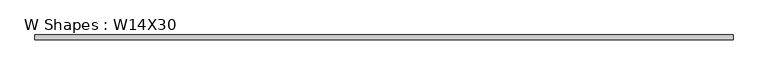
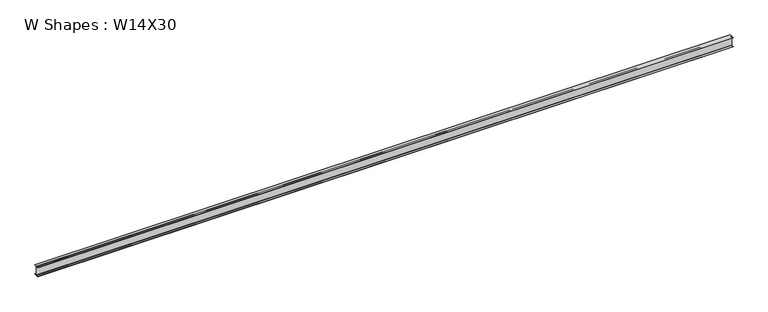
"""IFC4 building model written with IfcOpenShell, lengths in millimetres: beam geometry, W Shapes : W14X30."""

from ifc_helpers import new_model, si_unit, point, frame, frame_2d, origin, place, context, project, spatial, polyline, circle_curve, trimmed, segment, composite_curve, outline, extrude, source, transform, mapped, element, save


def w_shapes_w14x30_f0ef5163(model_context):
    return source(origin(), model_context, "Body", "SweptSolid", [
        extrude(outline(composite_curve([segment(polyline([(85.471, -165.481), (85.471, -175.26), (-85.471, -175.26), (-85.471, -165.481), (-13.589, -165.481)]), True, "CONTINUOUS"), segment(trimmed(circle_curve(frame_2d((-13.589, -155.321)), 10.16), [point((-13.589, -165.481))], [point((-3.429, -155.321))], True, "CARTESIAN"), True, "CONTINUOUS"), segment(polyline([(-3.429, -155.321), (-3.429, 155.321)]), True, "CONTINUOUS"), segment(trimmed(circle_curve(frame_2d((-13.589, 155.321)), 10.16), [point((-3.429, 155.321))], [point((-13.589, 165.481))], True, "CARTESIAN"), True, "CONTINUOUS"), segment(polyline([(-13.589, 165.481), (-85.471, 165.481), (-85.471, 175.26), (85.471, 175.26), (85.471, 165.481), (13.589, 165.481)]), True, "CONTINUOUS"), segment(trimmed(circle_curve(frame_2d((13.589, 155.321)), 10.16), [point((13.589, 165.481))], [point((3.429, 155.321))], True, "CARTESIAN"), True, "CONTINUOUS"), segment(polyline([(3.429, 155.321), (3.429, -155.321)]), True, "CONTINUOUS"), segment(trimmed(circle_curve(frame_2d((13.589, -155.321)), 10.16), [point((3.429, -155.321))], [point((13.589, -165.481))], True, "CARTESIAN"), True, "CONTINUOUS"), segment(polyline([(13.589, -165.481), (85.471, -165.481)]), True, "CONTINUOUS")], self_intersect=False)), frame((-12500.0, 0.0, 0.0), z_axis=(1.0, 0.0, 0.0), x_axis=(0.0, 1.0, 0.0)), (0.0, 0.0, 1.0), 25000.0),
    ])


if __name__ == "__main__":
    model = new_model("IFC4")
    model_context = context("Model", 3, world=origin())
    ifc_project = project(units=[si_unit("LENGTHUNIT", "METRE", prefix="MILLI")], contexts=[model_context])
    site = spatial("IfcSite", under=ifc_project)
    building = spatial("IfcBuilding", under=site)
    placement = place(None, origin())
    w_shapes_w14x30_shape = w_shapes_w14x30_f0ef5163(model_context)
    element("IfcBeam", 1, ObjectType="W Shapes : W14X30", at=placement, inside=building, context=model_context, shape_type="MappedRepresentation", body=[
        mapped(w_shapes_w14x30_shape, transform((0.0, 0.0, 0.0), x_axis=(1.0, 0.0, 0.0), y_axis=(0.0, 1.0, 0.0), z_axis=(0.0, 0.0, 1.0))),
    ])
    save(model, "model.ifc")

# Revit data of these elements
# Type "W Shapes : W14X30"
#   Section Name Key = "W14X30"
#   Width = 6.730"
#   Web Thickness = 0.270"
#   Web Fillet = 0.400"
#   Warping Constant = 887.00 in⁶
#   Torsional Moment of Inertia = 0.38 in⁴
#   Section Area = 8.85 in²
#   Plastic Modulus weak axis = 8.99 in³
#   Plastic Modulus strong axis = 47.30 in³
#   Perimeter = 4.441 ft²/ft
#   Nominal Weight = 30.00 lbf/ft
#   Moment of Inertia weak axis = 19.60 in⁴
#   Moment of Inertia strong axis = 291.00 in⁴
#   Height = 13.800"
#   Flange Thickness = 0.385"
#   Elastic Modulus weak axis = 5.82 in³
#   Elastic Modulus strong axis = 42.00 in³
#   Clear Web Height = 0' - 11 5/8"
#   Centroid Vertical = 6.900"
#   Centroid Horizontal = 3.365"
#   Bolt Spacing = 0' - 3 1/2"
#   Length [instance default] = 1524 mm
#   Structural Material [instance default] = Steel ASTM A992
#   Principal Axes Angle = 0
# Element 1 (IfcBeam, "W Shapes : W14X30")
#   Length = 25000 mm
#   Materials on its faces: "Steel ASTM A992"
# Materials
#   "Steel ASTM A992": class "Metal", colour RGB 199 199 199, transparency 0, Description = "Structural steel 50ksi", Cost = 0
